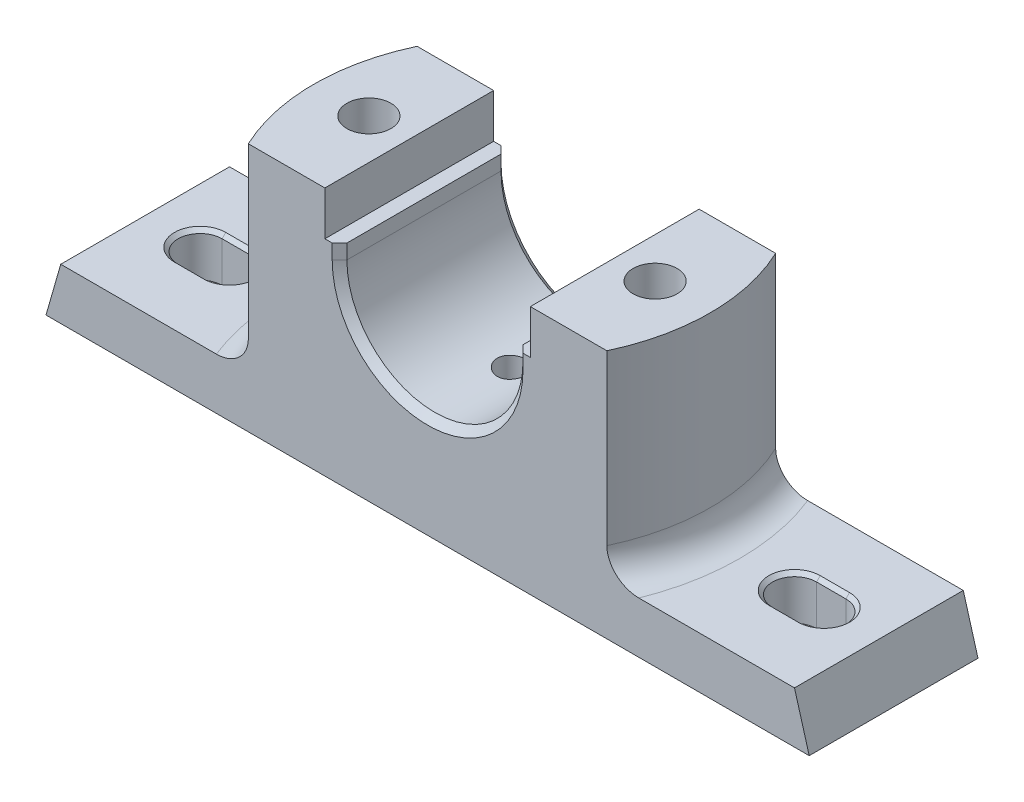
SolidWorks part; units mm, degrees
material "Plain Carbon Steel"
ref_plane "Front Plane" through (0, 0, 0) normal (0, 0, 1) x (1, 0, 0)
ref_plane "Top Plane" through (0, 0, 0) normal (0, 1, 0) x (1, 0, 0)
ref_plane "Right Plane" through (0, 0, 0) normal (1, 0, 0) x (0, 0, -1)
sketch "Base Plate Sketch" plane through (0, 0, 0) normal (0, 1, 0) x (1, 0, 0)
  line L1 (-104, 23) -> (104, 23)
  line L2 (-104, 23) -> (-104, -23)
  line L3 (-104, -23) -> (104, -23)
  line L4 (104, 23) -> (104, -23)
  line L5 (-104, 23) -> (104, -23) construction
  line L6 (-104, -23) -> (104, 23) construction
  point P0 (0, 0)
  dimension "D1" = 208
  dimension "D2" = 46
extrude "Base Plate 208x46x14" add sketch "Base Plate Sketch" along normal blind 14
sketch "Base End Bevel Sketch" plane through (0, 0, 23) normal (0, 0, 1) x (1, 0, 0)
  line L0 (-104, 0) -> (-99.9856, 14)
  line L1 (104, 0) -> (99.9856, 14)
  line L4 (-104, 0) -> (104, 0)
  line L5 (104, 0) -> (104, 14)
  line L6 (104, 14) -> (-104, 14)
  line L7 (-104, 14) -> (-104, 0)
  line L8 (-104, 0) -> (104, 0)
  line L10 (99.9856, 14) -> (-99.9856, 14)
  dimension "D2" = 106
  dimension "D3" = 106
  dimension "D1" = 0
extrude "Base End Bevels" cut sketch "Base End Bevel Sketch" against normal through all flip side to cut
sketch "Pedestal Sketch" plane through (0, 0, 23) normal (0, 0, 1) x (1, 0, 0)
  line L0 (-99.9856, 14) -> (99.9856, 14) construction
  line L1 (-56, 14) -> (56, 14)
  line L2 (-56, 14) -> (-56, 68)
  line L3 (-56, 68) -> (-28, 68)
  line L4 (-28, 68) -> (-28, 56)
  line L5 (-28, 56) -> (-24, 56)
  line L6 (-24, 56) -> (-24, 52)
  line L7 (0, -25.3) -> (0, 25.3) construction
  line L8 (28, 56) -> (24, 56)
  line L9 (24, 56) -> (24, 52)
  line L10 (28, 68) -> (28, 56)
  line L11 (56, 68) -> (28, 68)
  line L12 (56, 14) -> (56, 68)
  arc A0 (-24, 52) -> (24, 52) centre (0, 52) ccw
  dimension "D2" = 48
  dimension "D1" = 54
  dimension "D3" = 38
  dimension "D4" = 28
  dimension "D5" = 28
  dimension "D6" = 4
extrude "Bearing Pedestal" add sketch "Pedestal Sketch" against normal through all
sketch "Underside Relief Sketch" plane through (0, 0, 0) normal (0, -1, 0) x (1, 0, 0)
  line L0 (-104, 23) -> (104, 23) construction
  line L1 (-97.5, 18) -> (97.5, 18)
  line L2 (-97.5, 18) -> (-97.5, -18)
  line L3 (-97.5, -18) -> (97.5, -18)
  line L4 (97.5, 18) -> (97.5, -18)
  line L5 (-97.5, 18) -> (97.5, -18) construction
  line L6 (-97.5, -18) -> (97.5, 18) construction
  point P1 (0, 0)
  dimension "D1" = 195
  dimension "D2" = 5
extrude "Underside Relief 2mm" cut sketch "Underside Relief Sketch" against normal blind 2
sketch "Bearing Bore Sketch" plane through (0, 2, 0) normal (0, -1, 0) x (1, 0, 0)
  line L0 (0, -25.3) -> (0, 25.3) construction
  line L1 (25, 14) -> (53, 14)
  line L2 (25, 14) -> (25, -14)
  line L3 (25, -14) -> (53, -14)
  line L4 (53, 14) -> (53, -14)
  line L5 (25, 14) -> (53, -14) construction
  line L6 (25, -14) -> (53, 14) construction
  line L7 (-25, -14) -> (-53, -14)
  line L8 (-53, 14) -> (-53, -14)
  line L9 (-25, 14) -> (-53, 14)
  line L10 (-25, 14) -> (-25, -14)
  point P0 (39, 0)
  dimension "D1" = 39
  dimension "D2" = 28
  dimension "D3" = 28
extrude "Bearing Bore Cut" cut sketch "Bearing Bore Sketch" against normal blind 10
sketch "Mounting Slots Sketch" plane through (0, 0, 0) normal (0, 1, 0) x (1, 0, 0)
  line L0 (77, 0) -> (85, 0) construction
  line L1 (77, 6) -> (85, 6)
  line L2 (77, -6) -> (85, -6)
  line L3 (0, -25.3) -> (0, 25.3) construction
  line L4 (-77, 0) -> (-85, 0) construction
  line L5 (-77, 6) -> (-85, 6)
  line L6 (-77, -6) -> (-85, -6)
  arc A0 (77, 6) -> (77, -6) centre (77, 0) ccw
  arc A1 (85, -6) -> (85, 6) centre (85, 0) ccw
  arc A2 (-77, 6) -> (-77, -6) centre (-77, 0) cw
  arc A3 (-85, -6) -> (-85, 6) centre (-85, 0) cw
  point P3 (81, 0)
  point P13 (-81, 0)
  dimension "D2" = 6
  dimension "D1" = 8
  dimension "D3" = 77
extrude "Mounting Slots 2x8" cut sketch "Mounting Slots Sketch" along normal through all
hole_wizard "Cap Bolt Holes 2xØ12" positions "Sketch9" profile "Sketch10" hole size "Ø1.0" standard "ANSI Metric" end condition through all
sketch "Sketch9" plane through (0, 12, 0) normal (0, -1, 0) x (-1, 0, 0)
  point P0 (-39, 0)
  point P2 (39, 0)
  dimension "D1" = 39
  dimension "D2" = 78
sketch "Sketch10" plane through (39, 12, 0) normal (1, 0, 0) x (0, 0, -1)
  line L0 (0, 0) -> (0, 56)
  line L1 (0, 56) -> (6, 56)
  line L2 (6, 56) -> (6, 0)
  line L5 (6, 0) -> (0, 0)
  line L11 (0, -6.35) -> (0, 107.95) construction
  dimension "Thru Hole Dia." = 12
  dimension "Thru Hole Depth" = 56
chamfer "Pedestal Chamfer 2mm" distance 2 angle 45 6 edges at (24, 54, 23) (24, 54, -23) (-24, 54, 23) (-24, 54, -23) (0, 28, 23) (0, 28, -23)
chamfer "Slot Edge Chamfer 1mm" distance 1 angle 45 8 edges at (-81, 14, -6) (-71, 14, 0) (-91, 14, 0) (-81, 14, 6) (71, 14, 0) (81, 14, -6) (81, 14, 6) (91, 14, 0)
hole_wizard "Drilled Hole Ø8" positions "Sketch11" profile "Sketch13" hole size "Ø1.0" standard "ANSI Metric"
sketch "Sketch11" plane through (0, 56, 0) normal (0, 1, 0) x (1, 0, 0)
  point P0 (0, 0)
sketch "Sketch13" plane through (0, 56, 0) normal (1, 0, 0) x (0, 0, 1)
  line L0 (0, 0) -> (0, 36)
  line L1 (0, 36) -> (4, 36)
  line L2 (4, 36) -> (4, 0)
  line L5 (4, 0) -> (0, 0)
  line L10 (0, 36) -> (-4, 36) construction
  line L11 (0, -6.35) -> (0, 107.95) construction
  dimension "Hole Dia." = 8
  dimension "Hole Depth" = 36
  dimension "Drill Angle" = 180
sketch "Pedestal Profile Sketch" plane through (0, 68, 0) normal (0, 1, 0) x (1, 0, 0)
  line L0 (0, -25.3) -> (0, 25.3) construction
  line L4 (-56, -23) -> (-28, -23)
  line L5 (-28, -23) -> (-28, 23)
  line L6 (-28, 23) -> (-56, 23)
  line L7 (-56, 23) -> (-56, -23)
  line L8 (-56, -23) -> (-48.8569, -23)
  line L10 (-48.8569, 23) -> (-56, 23)
  line L11 (-56, 23) -> (-56, -23)
  line L12 (28, -23) -> (56, -23)
  line L13 (56, -23) -> (56, 23)
  line L14 (56, 23) -> (28, 23)
  line L15 (28, 23) -> (28, -23)
  line L16 (48.8569, -23) -> (56, -23)
  line L17 (56, -23) -> (56, 23)
  line L18 (56, 23) -> (48.8569, 23)
  arc A0 (48.8569, -23) -> (48.8569, 23) centre (0, 0) ccw
  arc A1 (-48.8569, -23) -> (-48.8569, 23) centre (0, 0) cw
  dimension "D3" = 54
  dimension "D1" = 0
  dimension "D2" = 0
extrude "Pedestal Profile Cut" cut sketch "Pedestal Profile Sketch" against normal blind 54
fillet "Pedestal Base Fillet R8" radius 8 2 edges at (54, 14, 0) (-54, 14, 0)
